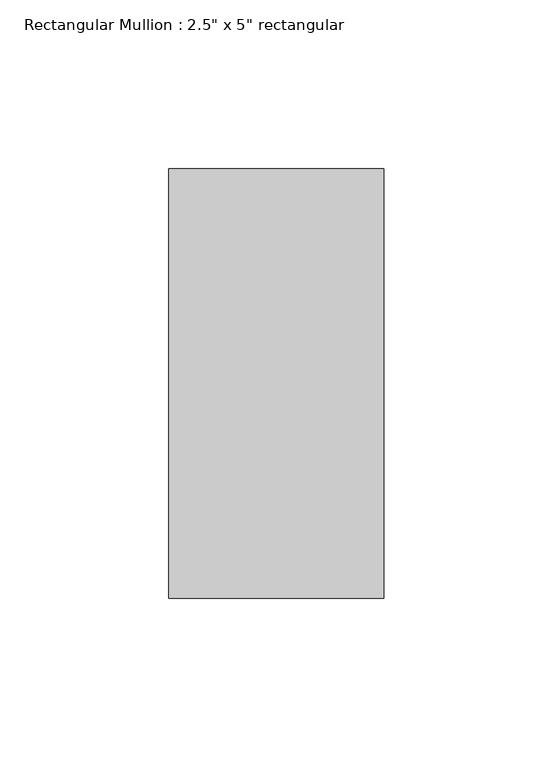
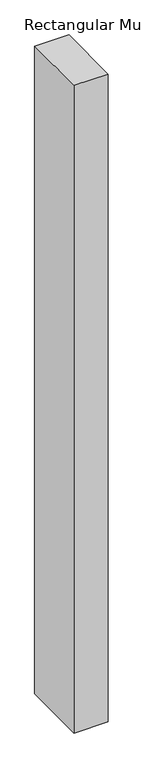
"""IFC4 building model written with IfcOpenShell, lengths in millimetres: member geometry."""

from ifc_helpers import new_model, si_unit, frame, origin, place, context, project, spatial, polyline, outline, extrude, source, transform, mapped, element, save


def member_9ae880e2(model_context):
    return source(origin(), model_context, "Body", "SweptSolid", [
        extrude(outline(polyline([(0.0, 63.5), (0.0, -63.5), (-63.5, -63.5), (-63.5, 63.5), (0.0, 63.5)])), frame((0.0, 0.0, -1274.1056645), z_axis=(0.0, 0.0, 1.0), x_axis=(1.0, 0.0, 0.0)), (0.0, 0.0, 1.0), 1274.1056645),
    ])


if __name__ == "__main__":
    model = new_model("IFC4")
    model_context = context("Model", 3, world=origin())
    ifc_project = project(units=[si_unit("LENGTHUNIT", "METRE", prefix="MILLI")], contexts=[model_context])
    site = spatial("IfcSite", under=ifc_project)
    building = spatial("IfcBuilding", under=site)
    placement = place(None, origin())
    member_shape = member_9ae880e2(model_context)
    element("IfcMember", 1, ObjectType="Rectangular Mullion : 2.5\" x 5\" rectangular", at=placement, inside=building, context=model_context, shape_type="MappedRepresentation", body=[
        mapped(member_shape, transform((0.0, 0.0, 0.0), x_axis=(1.0, 0.0, 0.0), y_axis=(0.0, 1.0, 0.0), z_axis=(0.0, 0.0, 1.0))),
    ])
    save(model, "model.ifc")

# Revit data of these elements
# Type "Rectangular Mullion : 2.5\" x 5\" rectangular"
#   built-in parameter 1007304 = 0.416667 (stored number, unit not read)
#   built-in parameter 1007301 = 0.104167 (stored number, unit not read)
#   built-in parameter 1007300 = 0.104167 (stored number, unit not read)
